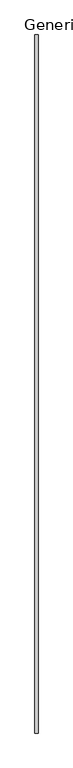
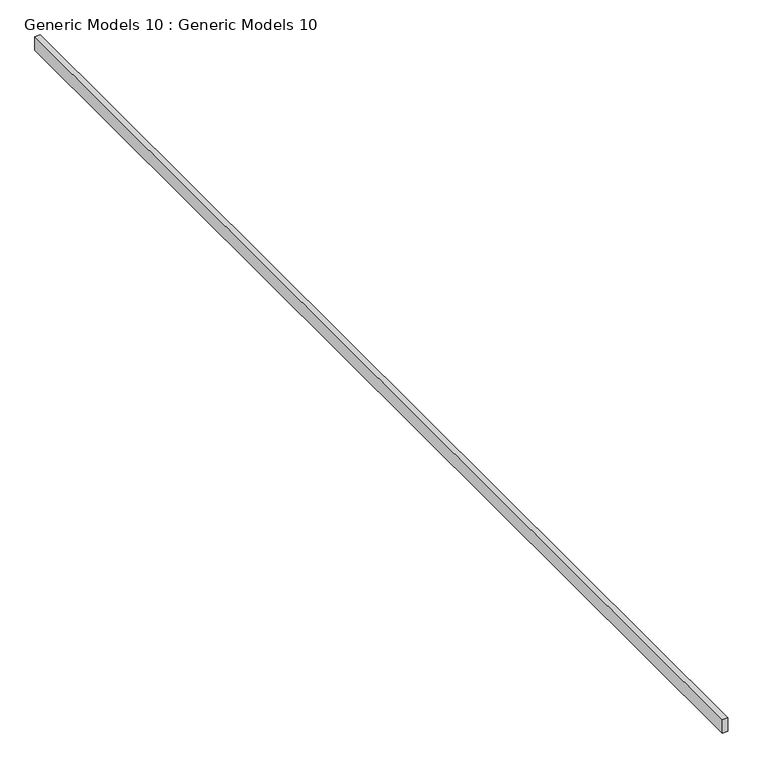
"""IFC4 building model written with IfcOpenShell, lengths in millimetres: proxy geometry, Generic Models 10 : Generic Models 10."""

from ifc_helpers import new_model, si_unit, frame, origin, place, context, project, spatial, polyline, outline, extrude, source, transform, mapped, element, save


def generic_models_10_generic_models_10_d49a56e1(model_context):
    return source(origin(), model_context, "Body", "SweptSolid", [
        extrude(outline(polyline([(10213.9846336, 10069.2926686), (10213.9846336, -6998.6262311), (10137.9423568, -6998.6262311), (10137.9423568, 10069.2926686), (10213.9846336, 10069.2926686)])), frame((0.0, 0.0, 6198.4771746), z_axis=(0.0, 0.0, 1.0), x_axis=(1.0, 0.0, 0.0)), (0.0, 0.0, 1.0), 202.3228254),
    ])


if __name__ == "__main__":
    model = new_model("IFC4")
    model_context = context("Model", 3, world=origin())
    ifc_project = project(units=[si_unit("LENGTHUNIT", "METRE", prefix="MILLI")], contexts=[model_context])
    site = spatial("IfcSite", under=ifc_project)
    building = spatial("IfcBuilding", under=site)
    placement = place(None, origin())
    generic_models_10_generic_models_10_shape = generic_models_10_generic_models_10_d49a56e1(model_context)
    element("IfcBuildingElementProxy", 1, Name="Generic Models 10 : Generic Models 10", ObjectType="Generic Models 10 : Generic Models 10", at=placement, inside=building, context=model_context, shape_type="MappedRepresentation", body=[
        mapped(generic_models_10_generic_models_10_shape, transform((0.0, 0.0, 0.0), x_axis=(1.0, 0.0, 0.0), y_axis=(0.0, 1.0, 0.0), z_axis=(0.0, 0.0, 1.0))),
    ])
    save(model, "model.ifc")

# Revit data of these elements
# Element 1 (IfcBuildingElementProxy, "Generic Models 10 : Generic Models 10")
#   Materials on its faces: "Clad - White"
# Materials
#   "Clad - White": class "Wood", colour RGB 242 242 238, transparency 0, Cost = 0
